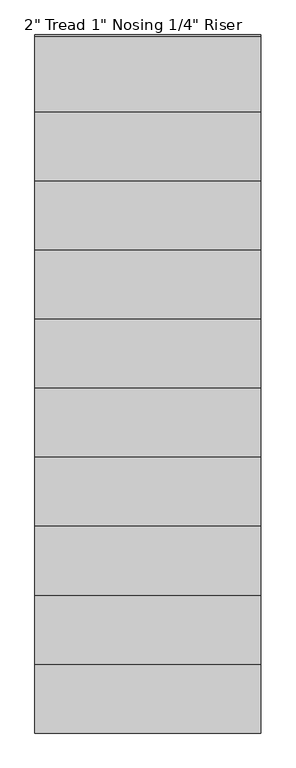
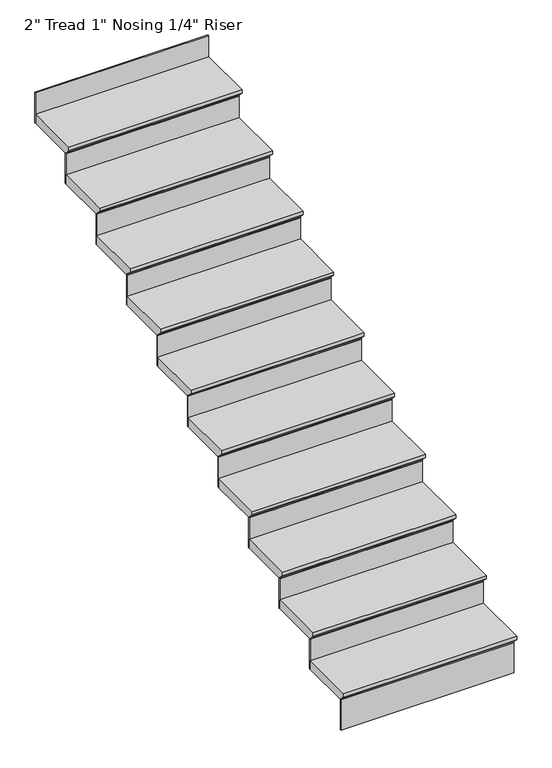
"""IFC4 building model written with IfcOpenShell, lengths in millimetres: stair flight geometry."""

from ifc_helpers import new_model, si_unit, frame, origin, place, context, project, spatial, polyline, outline, extrude, source, transform, mapped, element, save


def stair_flight_c801c68a(model_context):
    return source(origin(), model_context, "Body", "SweptSolid", [
        extrude(outline(polyline([(-2391.1272484, 1659.4666667), (-2086.3272484, 1659.4666667), (-2086.3272484, 1608.6666667), (-2365.7272484, 1608.6666667), (-2365.7272484, 1615.0166667), (-2391.1272484, 1640.4166667), (-2391.1272484, 1659.4666667)])), frame((-5951.5750936, 0.0, 0.0), z_axis=(1.0, 0.0, 0.0), x_axis=(0.0, 1.0, 0.0)), (0.0, 0.0, 1.0), 914.4),
        extrude(outline(polyline([(-5037.1750936, -2359.3772484), (-5037.1750936, -2365.7272484), (-5951.5750936, -2365.7272484), (-5951.5750936, -2359.3772484), (-5037.1750936, -2359.3772484)])), frame((0.0, 0.0, 1439.3333333), z_axis=(0.0, 0.0, 1.0), x_axis=(1.0, 0.0, 0.0)), (0.0, 0.0, 1.0), 169.3333333),
        extrude(outline(polyline([(-5037.1750936, -2079.9772484), (-5037.1750936, -2086.3272484), (-5951.5750936, -2086.3272484), (-5951.5750936, -2079.9772484), (-5037.1750936, -2079.9772484)])), frame((0.0, 0.0, 1608.6666667), z_axis=(0.0, 0.0, 1.0), x_axis=(1.0, 0.0, 0.0)), (0.0, 0.0, 1.0), 169.3333333),
        extrude(outline(polyline([(-2111.7272484, 1828.8), (-1806.9272484, 1828.8), (-1806.9272484, 1778.0), (-2086.3272484, 1778.0), (-2086.3272484, 1784.35), (-2111.7272484, 1809.75), (-2111.7272484, 1828.8)])), frame((-5951.5750936, 0.0, 0.0), z_axis=(1.0, 0.0, 0.0), x_axis=(0.0, 1.0, 0.0)), (0.0, 0.0, 1.0), 914.4),
        extrude(outline(polyline([(-5037.1750936, -1800.5772484), (-5037.1750936, -1806.9272484), (-5951.5750936, -1806.9272484), (-5951.5750936, -1800.5772484), (-5037.1750936, -1800.5772484)])), frame((0.0, 0.0, 1778.0), z_axis=(0.0, 0.0, 1.0), x_axis=(1.0, 0.0, 0.0)), (0.0, 0.0, 1.0), 169.3333333),
        extrude(outline(polyline([(-1832.3272484, 1998.1333333), (-1527.5272484, 1998.1333333), (-1527.5272484, 1947.3333333), (-1806.9272484, 1947.3333333), (-1806.9272484, 1953.6833333), (-1832.3272484, 1979.0833333), (-1832.3272484, 1998.1333333)])), frame((-5951.5750936, 0.0, 0.0), z_axis=(1.0, 0.0, 0.0), x_axis=(0.0, 1.0, 0.0)), (0.0, 0.0, 1.0), 914.4),
        extrude(outline(polyline([(-5037.1750936, -1521.1772484), (-5037.1750936, -1527.5272484), (-5951.5750936, -1527.5272484), (-5951.5750936, -1521.1772484), (-5037.1750936, -1521.1772484)])), frame((0.0, 0.0, 1947.3333333), z_axis=(0.0, 0.0, 1.0), x_axis=(1.0, 0.0, 0.0)), (0.0, 0.0, 1.0), 169.3333333),
        extrude(outline(polyline([(-1552.9272484, 2167.4666667), (-1248.1272484, 2167.4666667), (-1248.1272484, 2116.6666667), (-1527.5272484, 2116.6666667), (-1527.5272484, 2123.0166667), (-1552.9272484, 2148.4166667), (-1552.9272484, 2167.4666667)])), frame((-5951.5750936, 0.0, 0.0), z_axis=(1.0, 0.0, 0.0), x_axis=(0.0, 1.0, 0.0)), (0.0, 0.0, 1.0), 914.4),
        extrude(outline(polyline([(-5037.1750936, -1241.7772484), (-5037.1750936, -1248.1272484), (-5951.5750936, -1248.1272484), (-5951.5750936, -1241.7772484), (-5037.1750936, -1241.7772484)])), frame((0.0, 0.0, 2116.6666667), z_axis=(0.0, 0.0, 1.0), x_axis=(1.0, 0.0, 0.0)), (0.0, 0.0, 1.0), 169.3333333),
        extrude(outline(polyline([(-1273.5272484, 2336.8), (-968.7272484, 2336.8), (-968.7272484, 2286.0), (-1248.1272484, 2286.0), (-1248.1272484, 2292.35), (-1273.5272484, 2317.75), (-1273.5272484, 2336.8)])), frame((-5951.5750936, 0.0, 0.0), z_axis=(1.0, 0.0, 0.0), x_axis=(0.0, 1.0, 0.0)), (0.0, 0.0, 1.0), 914.4),
        extrude(outline(polyline([(-5037.1750936, -962.3772484), (-5037.1750936, -968.7272484), (-5951.5750936, -968.7272484), (-5951.5750936, -962.3772484), (-5037.1750936, -962.3772484)])), frame((0.0, 0.0, 2286.0), z_axis=(0.0, 0.0, 1.0), x_axis=(1.0, 0.0, 0.0)), (0.0, 0.0, 1.0), 169.3333333),
        extrude(outline(polyline([(-994.1272484, 2506.1333333), (-689.3272484, 2506.1333333), (-689.3272484, 2455.3333333), (-968.7272484, 2455.3333333), (-968.7272484, 2461.6833333), (-994.1272484, 2487.0833333), (-994.1272484, 2506.1333333)])), frame((-5951.5750936, 0.0, 0.0), z_axis=(1.0, 0.0, 0.0), x_axis=(0.0, 1.0, 0.0)), (0.0, 0.0, 1.0), 914.4),
        extrude(outline(polyline([(-5037.1750936, -682.9772484), (-5037.1750936, -689.3272484), (-5951.5750936, -689.3272484), (-5951.5750936, -682.9772484), (-5037.1750936, -682.9772484)])), frame((0.0, 0.0, 2455.3333333), z_axis=(0.0, 0.0, 1.0), x_axis=(1.0, 0.0, 0.0)), (0.0, 0.0, 1.0), 169.3333333),
        extrude(outline(polyline([(-714.7272484, 2675.4666667), (-409.9272484, 2675.4666667), (-409.9272484, 2624.6666667), (-689.3272484, 2624.6666667), (-689.3272484, 2631.0166667), (-714.7272484, 2656.4166667), (-714.7272484, 2675.4666667)])), frame((-5951.5750936, 0.0, 0.0), z_axis=(1.0, 0.0, 0.0), x_axis=(0.0, 1.0, 0.0)), (0.0, 0.0, 1.0), 914.4),
        extrude(outline(polyline([(-5037.1750936, -403.5772484), (-5037.1750936, -409.9272484), (-5951.5750936, -409.9272484), (-5951.5750936, -403.5772484), (-5037.1750936, -403.5772484)])), frame((0.0, 0.0, 2624.6666667), z_axis=(0.0, 0.0, 1.0), x_axis=(1.0, 0.0, 0.0)), (0.0, 0.0, 1.0), 169.3333333),
        extrude(outline(polyline([(-435.3272484, 2844.8), (-130.5272484, 2844.8), (-130.5272484, 2794.0), (-409.9272484, 2794.0), (-409.9272484, 2800.35), (-435.3272484, 2825.75), (-435.3272484, 2844.8)])), frame((-5951.5750936, 0.0, 0.0), z_axis=(1.0, 0.0, 0.0), x_axis=(0.0, 1.0, 0.0)), (0.0, 0.0, 1.0), 914.4),
        extrude(outline(polyline([(-5037.1750936, -124.1772484), (-5037.1750936, -130.5272484), (-5951.5750936, -130.5272484), (-5951.5750936, -124.1772484), (-5037.1750936, -124.1772484)])), frame((0.0, 0.0, 2794.0), z_axis=(0.0, 0.0, 1.0), x_axis=(1.0, 0.0, 0.0)), (0.0, 0.0, 1.0), 169.3333333),
        extrude(outline(polyline([(-155.9272484, 3014.1333333), (148.8727516, 3014.1333333), (148.8727516, 2963.3333333), (-130.5272484, 2963.3333333), (-130.5272484, 2969.6833333), (-155.9272484, 2995.0833333), (-155.9272484, 3014.1333333)])), frame((-5951.5750936, 0.0, 0.0), z_axis=(1.0, 0.0, 0.0), x_axis=(0.0, 1.0, 0.0)), (0.0, 0.0, 1.0), 914.4),
        extrude(outline(polyline([(-5037.1750936, 155.2227516), (-5037.1750936, 148.8727516), (-5951.5750936, 148.8727516), (-5951.5750936, 155.2227516), (-5037.1750936, 155.2227516)])), frame((0.0, 0.0, 2963.3333333), z_axis=(0.0, 0.0, 1.0), x_axis=(1.0, 0.0, 0.0)), (0.0, 0.0, 1.0), 169.3333333),
        extrude(outline(polyline([(-5037.1750936, 434.6227516), (-5037.1750936, 428.2727516), (-5951.5750936, 428.2727516), (-5951.5750936, 434.6227516), (-5037.1750936, 434.6227516)])), frame((0.0, 0.0, 3132.6666667), z_axis=(0.0, 0.0, 1.0), x_axis=(1.0, 0.0, 0.0)), (0.0, 0.0, 1.0), 169.3333333),
        extrude(outline(polyline([(123.4727516, 3183.4666667), (428.2727516, 3183.4666667), (428.2727516, 3132.6666667), (148.8727516, 3132.6666667), (148.8727516, 3139.0166667), (123.4727516, 3164.4166667), (123.4727516, 3183.4666667)])), frame((-5951.5750936, 0.0, 0.0), z_axis=(1.0, 0.0, 0.0), x_axis=(0.0, 1.0, 0.0)), (0.0, 0.0, 1.0), 914.4),
    ])


if __name__ == "__main__":
    model = new_model("IFC4")
    model_context = context("Model", 3, world=origin())
    ifc_project = project(units=[si_unit("LENGTHUNIT", "METRE", prefix="MILLI")], contexts=[model_context])
    site = spatial("IfcSite", under=ifc_project)
    building = spatial("IfcBuilding", under=site)
    placement = place(None, origin())
    stair_flight_shape = stair_flight_c801c68a(model_context)
    element("IfcStairFlight", 1, ObjectType="2\" Tread 1\" Nosing 1/4\" Riser", at=placement, inside=building, context=model_context, shape_type="MappedRepresentation", body=[
        mapped(stair_flight_shape, transform((0.0, 0.0, 0.0), x_axis=(1.0, 0.0, 0.0), y_axis=(0.0, 1.0, 0.0), z_axis=(0.0, 0.0, 1.0))),
    ])
    save(model, "model.ifc")
